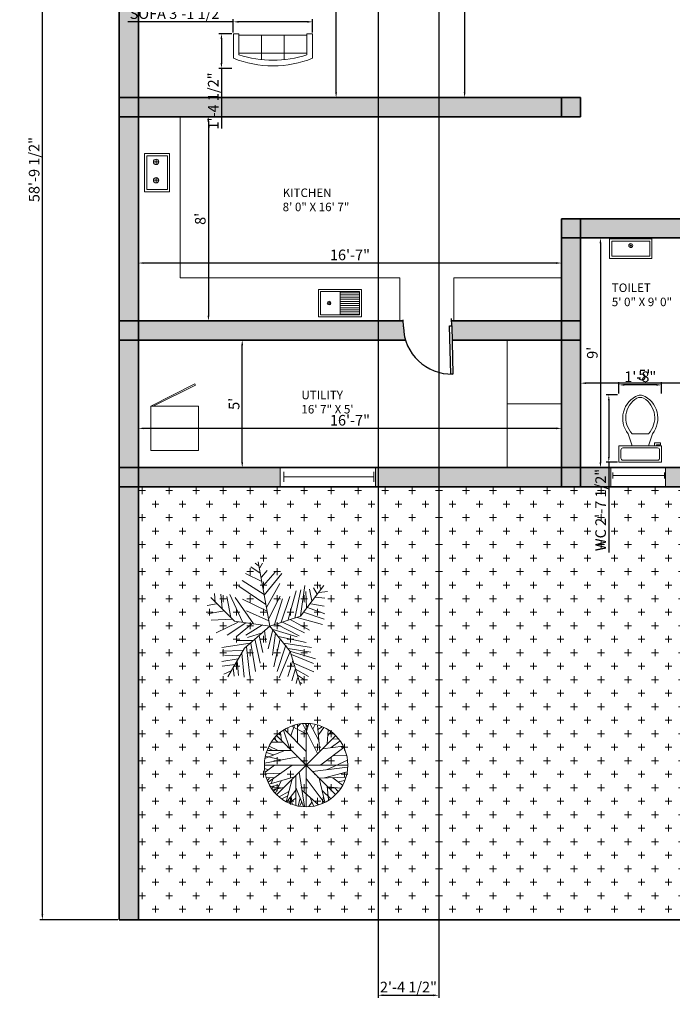
# Model space of a CAD drawing. Units: millimetres. Extents: x 2768 to 4359, y 795 to 1583.
# Tile 6 of 13: x 3572 to 3880, y 795 to 1258. Entities that reach past the tile are written whole.
import ezdxf

# ---------------------------------------------------------------- set-up
doc = ezdxf.new("R2010")
doc.units = ezdxf.units.MM
for name, color, linetype, lineweight in [('A-ANNO-DIMS', 90, 'Continuous', 18), ('A-AREA-IDEN', 190, 'Continuous', 18), ('A-EQPM', 50, 'Continuous', 18), ('A-FLOR-CASE', 50, 'Continuous', 18), ('A-FLOR-FIXT', 50, 'Continuous', 18), ('A-FLOR-FIXT-PATT', 50, 'Continuous', 13), ('A-WALL-PATT', 140, 'Continuous', 9), ('doors', 10, 'Continuous', 25), ('furniture', 50, 'Continuous', 18), ('GARDEN', 109, 'Continuous', 18), ('L-PLNT-PATT', 109, 'Continuous', 13), ('walls', 140, 'Continuous', 35), ('windows', 30, 'Continuous', 18)]:
    doc.layers.add(name, color=color, linetype=linetype, lineweight=lineweight)
doc.styles.get("Standard").update_dxf_attribs({"font": 'arial.ttf'})
doc.dimstyles.new('ISO-25', dxfattribs={"dimtxt": 5, "dimasz": 2.5, "dimexe": 1.25, "dimexo": 0.625, "dimtad": 1, "dimdec": 0, "dimlunit": 3, "dimtxsty": 'Standard', "dimcen": 2.5, "dimadec": 0, "dimazin": 0, "dimtfac": 1, "dimtdec": 0, "dimtmove": 0, "dimatfit": 3, "dimfxl": 1, "dimarcsym": 0})

# ---------------------------------------------------------------- blocks, each defined once
blk = doc.blocks.new('*U38')
for p, q in [((0, 4), (0, 0)), ((0, 2), (36, 2)), ((36, 4), (36, 0))]:
    blk.add_line(p, q)
blk = doc.blocks.new('*U39')
for p, q in [((0, 4), (0, 0)), ((36, 4), (36, 0)), ((0, 2), (36, 2))]:
    blk.add_line(p, q)
blk = doc.blocks.new('Sofa - Roundback 7 ft.')
for p, q in [((-12.00002, -32.4421), (-12.00003, -6.5971)), ((11.99997, -32.4421), (11.99998, -6.5971)), ((-36.000027, -34), (-36.000027, -11.4696)), ((-35.999844, -13.3819), (35.9998, -13.3819)), ((35.99998, -34), (35.99998, -11.4696)), ((-36.000027, -32.4421), (35.99998, -32.4421))]:
    blk.add_line(p, q)
for points in [[(-36.000027, -34), (-42.000027, -34), (-42.000027, -8)], [(41.99998, -8), (41.99998, -34), (35.99998, -34)]]:
    blk.add_lwpolyline(points)
for centre, radius, start, end in [((0, -114.25), 114.25, 68.43141, 111.5686), ((-0.00001, -127.1968), 121.1968, 72.72033, 107.2797)]:
    blk.add_arc(centre, radius, start, end)
blk = doc.blocks.new('Toilet - top')
for p, q in [((9.5, -6), (9.5, -2)), ((-10, -8.5), (-8, -8.5)), ((-10, -9.5), (-10, -8.5)), ((-7, -9.5), (-10, -9.5)), ((-8, -8.5), (-8, -8)), ((-7, -8), (-7, -9.5)), ((-4, -8), (-6, -14)), ((4, -8), (6, -14)), ((4, -14), (-4, -14))]:
    blk.add_line(p, q)
blk.add_lwpolyline([(10.5, -8), (10.5, 0), (-10.5, 0), (-10.5, -8)], close=True)
for points in [[(-9.5, -2), (-9.5, -6)], [(8.5, -1), (-8.5, -1)], [(-8.5, -7), (8.5, -7)]]:
    blk.add_lwpolyline(points)
for centre, radius, start, end in [((-8.62, -1.88), 0.884, 81.8699, 188.1301), ((8.62, -1.88), 0.884, 351.8699, 98.1301), ((-8.62, -6.12), 0.884, 171.8699, 278.1301), ((8.62, -6.12), 0.884, 261.8699, 8.1301), ((3.52, -21.58), 12.17, 141.4691, 247.9714), ((4.2, -21.82), 11.33, 136.3677, 238.9468), ((-3.52, -21.58), 12.17, 292.0284, 38.5307), ((-4.2, -21.82), 11.33, 301.053, 43.6321), ((0, -27.88), 4, 245.7318, 294.2682), ((0, -29), 4, 254.8605, 285.1395)]:
    blk.add_arc(centre, radius, start, end)
blk = doc.blocks.new('*U2')
for p, q in [((0, 0), (0, -6)), ((40, 0), (40, -6))]:
    blk.add_line(p, q)
blk.add_lwpolyline([(0, 0), (0, 40), (1.75, 40), (1.75, 0)], close=True)
blk.add_arc((0, 0), 40, 0, 90)
blk = doc.blocks.new('*D50')
at = {"layer": 'A-ANNO-DIMS', "color": 0, "lineweight": -2, "transparency": 16777216}
for p, q in [((3727.24, 1378.81), (3720.1, 1378.81)), ((3721.35, 1224.31), (3721.35, 1376.31)), ((3727.24, 1221.81), (3720.1, 1221.81))]:
    blk.add_line(p, q, dxfattribs=at)
at = {"layer": 'A-ANNO-DIMS', "color": 0, "transparency": 16777216}
for points in [[(3720.94, 1376.31), (3721.77, 1376.31), (3721.35, 1378.81)], [(3720.94, 1224.31), (3721.77, 1224.31), (3721.35, 1221.81)]]:
    blk.add_solid(points, dxfattribs=at)
at = {"layer": 'Defpoints', "color": 0, "transparency": 16777216}
for p in [(3721.35, 1378.81), (3727.87, 1378.81), (3727.87, 1221.81)]:
    blk.add_point(p, dxfattribs=at)
at = {"layer": 'A-ANNO-DIMS', "color": 0, "transparency": 16777216, "insert": (3718.17, 1300.31), "char_height": 5, "attachment_point": 5, "rotation": 90}
blk.add_mtext('13\'-1"', dxfattribs=at)
blk = doc.blocks.new('*D51')
at = {"layer": 'A-ANNO-DIMS', "color": 0, "lineweight": -2, "transparency": 16777216}
for p, q in [((3628.37, 1143.84), (3628.37, 1142.77)), ((3824.87, 1144.02), (3630.87, 1144.02)), ((3827.37, 1143.84), (3827.37, 1142.77))]:
    blk.add_line(p, q, dxfattribs=at)
at = {"layer": 'A-ANNO-DIMS', "color": 0, "transparency": 16777216}
for points in [[(3630.87, 1144.44), (3630.87, 1143.61), (3628.37, 1144.02)], [(3824.87, 1144.44), (3824.87, 1143.61), (3827.37, 1144.02)]]:
    blk.add_solid(points, dxfattribs=at)
at = {"layer": 'Defpoints', "color": 0, "transparency": 16777216}
for p in [(3628.37, 1144.47), (3628.37, 1144.02), (3827.37, 1144.47)]:
    blk.add_point(p, dxfattribs=at)
at = {"layer": 'A-ANNO-DIMS', "color": 0, "transparency": 16777216, "insert": (3727.87, 1147.2), "char_height": 5, "attachment_point": 5}
blk.add_mtext('16\'-7"', dxfattribs=at)
blk = doc.blocks.new('*D52')
at = {"layer": 'A-ANNO-DIMS', "color": 0, "lineweight": -2, "transparency": 16777216}
for p, q in [((3661.29, 1210.31), (3661.29, 1119.31)), ((3661.92, 1212.81), (3662.54, 1212.81)), ((3661.92, 1116.81), (3662.54, 1116.81))]:
    blk.add_line(p, q, dxfattribs=at)
at = {"layer": 'A-ANNO-DIMS', "color": 0, "transparency": 16777216}
for points in [[(3660.87, 1210.31), (3661.71, 1210.31), (3661.29, 1212.81)], [(3660.87, 1119.31), (3661.71, 1119.31), (3661.29, 1116.81)]]:
    blk.add_solid(points, dxfattribs=at)
at = {"layer": 'Defpoints', "color": 0, "transparency": 16777216}
for p in [(3661.29, 1212.81), (3661.29, 1116.81), (3661.29, 1116.81)]:
    blk.add_point(p, dxfattribs=at)
at = {"layer": 'A-ANNO-DIMS', "color": 0, "transparency": 16777216, "insert": (3658.11, 1164.81), "char_height": 5, "attachment_point": 5, "rotation": 90}
blk.add_mtext("8'", dxfattribs=at)
blk = doc.blocks.new('*D53')
at = {"layer": 'A-ANNO-DIMS', "color": 0, "lineweight": -2, "transparency": 16777216}
for p, q in [((3678.21, 1107.81), (3675.93, 1107.81)), ((3677.18, 1050.31), (3677.18, 1105.31)), ((3678.21, 1047.81), (3675.93, 1047.81))]:
    blk.add_line(p, q, dxfattribs=at)
at = {"layer": 'A-ANNO-DIMS', "color": 0, "transparency": 16777216}
for points in [[(3676.76, 1105.31), (3677.6, 1105.31), (3677.18, 1107.81)], [(3676.76, 1050.31), (3677.6, 1050.31), (3677.18, 1047.81)]]:
    blk.add_solid(points, dxfattribs=at)
at = {"layer": 'Defpoints', "color": 0, "transparency": 16777216}
for p in [(3677.18, 1107.81), (3678.84, 1107.81), (3678.84, 1047.81)]:
    blk.add_point(p, dxfattribs=at)
at = {"layer": 'A-ANNO-DIMS', "color": 0, "transparency": 16777216, "insert": (3674.01, 1077.81), "char_height": 5, "attachment_point": 5, "rotation": 90}
blk.add_mtext("5'", dxfattribs=at)
blk = doc.blocks.new('*D54')
at = {"layer": 'A-ANNO-DIMS', "color": 0, "lineweight": -2, "transparency": 16777216}
for p, q in [((3628.37, 1062.14), (3628.37, 1067.52)), ((3824.87, 1066.27), (3630.87, 1066.27)), ((3827.37, 1062.14), (3827.37, 1067.52))]:
    blk.add_line(p, q, dxfattribs=at)
at = {"layer": 'A-ANNO-DIMS', "color": 0, "transparency": 16777216}
for points in [[(3630.87, 1066.69), (3630.87, 1065.85), (3628.37, 1066.27)], [(3824.87, 1066.69), (3824.87, 1065.85), (3827.37, 1066.27)]]:
    blk.add_solid(points, dxfattribs=at)
at = {"layer": 'Defpoints', "color": 0, "transparency": 16777216}
for p in [(3628.37, 1066.27), (3628.37, 1061.52), (3827.37, 1061.52)]:
    blk.add_point(p, dxfattribs=at)
at = {"layer": 'A-ANNO-DIMS', "color": 0, "transparency": 16777216, "insert": (3727.87, 1069.45), "char_height": 5, "attachment_point": 5}
blk.add_mtext('16\'-7"', dxfattribs=at)
blk = doc.blocks.new('*D55')
at = {"layer": 'A-ANNO-DIMS', "color": 0, "lineweight": -2, "transparency": 16777216}
for p, q in [((3843.53, 1155.81), (3846.96, 1155.81)), ((3845.71, 1153.31), (3845.71, 1050.31)), ((3843.53, 1047.81), (3846.96, 1047.81))]:
    blk.add_line(p, q, dxfattribs=at)
at = {"layer": 'A-ANNO-DIMS', "color": 0, "transparency": 16777216}
for points in [[(3845.29, 1153.31), (3846.13, 1153.31), (3845.71, 1155.81)], [(3845.29, 1050.31), (3846.13, 1050.31), (3845.71, 1047.81)]]:
    blk.add_solid(points, dxfattribs=at)
at = {"layer": 'Defpoints', "color": 0, "transparency": 16777216}
for p in [(3842.9, 1155.81), (3842.9, 1047.81), (3845.71, 1047.81)]:
    blk.add_point(p, dxfattribs=at)
at = {"layer": 'A-ANNO-DIMS', "color": 0, "transparency": 16777216, "insert": (3842.53, 1101.81), "char_height": 5, "attachment_point": 5, "rotation": 90}
blk.add_mtext("9'", dxfattribs=at)
blk = doc.blocks.new('*D56')
at = {"layer": 'A-ANNO-DIMS', "color": 0, "lineweight": -2, "transparency": 16777216}
for p, q in [((3836.37, 1089), (3836.37, 1086.28)), ((3896.37, 1089), (3896.37, 1086.28)), ((3893.87, 1087.53), (3838.87, 1087.53))]:
    blk.add_line(p, q, dxfattribs=at)
at = {"layer": 'A-ANNO-DIMS', "color": 0, "transparency": 16777216}
for points in [[(3838.87, 1087.95), (3838.87, 1087.12), (3836.37, 1087.53)], [(3893.87, 1087.95), (3893.87, 1087.12), (3896.37, 1087.53)]]:
    blk.add_solid(points, dxfattribs=at)
at = {"layer": 'Defpoints', "color": 0, "transparency": 16777216}
for p in [(3836.37, 1089.62), (3896.37, 1089.62), (3836.37, 1087.53)]:
    blk.add_point(p, dxfattribs=at)
at = {"layer": 'A-ANNO-DIMS', "color": 0, "transparency": 16777216, "insert": (3866.37, 1090.7), "char_height": 5, "attachment_point": 5}
blk.add_mtext("5'", dxfattribs=at)
blk = doc.blocks.new('*D65')
at = {"layer": 'A-ANNO-DIMS', "color": 0, "lineweight": -2, "transparency": 16777216}
for p, q in [((3776.14, 1378.81), (3783.06, 1378.81)), ((3781.81, 1376.31), (3781.81, 1224.31)), ((3776.14, 1221.81), (3783.06, 1221.81))]:
    blk.add_line(p, q, dxfattribs=at)
at = {"layer": 'A-ANNO-DIMS', "color": 0, "transparency": 16777216}
for points in [[(3781.39, 1376.31), (3782.23, 1376.31), (3781.81, 1378.81)], [(3781.39, 1224.31), (3782.23, 1224.31), (3781.81, 1221.81)]]:
    blk.add_solid(points, dxfattribs=at)
at = {"layer": 'Defpoints', "color": 0, "transparency": 16777216}
for p in [(3775.51, 1378.81), (3775.51, 1221.81), (3781.81, 1221.81)]:
    blk.add_point(p, dxfattribs=at)
at = {"layer": 'A-ANNO-DIMS', "color": 0, "transparency": 16777216, "insert": (3778.63, 1300.31), "char_height": 5, "attachment_point": 5, "rotation": 90}
blk.add_mtext('13\'-1"', dxfattribs=at)
blk = doc.blocks.new('*U70')
for p, q in [((-8.737, 47.138), (-17.069, 52.711)), ((-10.186, 53.64), (-13.084, 55.962)), ((0, 0), (-10.5, 57)), ((-9.099, 51.782), (-6.563, 55.962)), ((-7.288, 39.707), (-21.778, 46.673)), ((-7.65, 43.423), (-2.578, 49.46)), ((-5.839, 35.992), (4.667, 48.067)), ((-5.114, 27.632), (10.463, 46.673)), ((-3.665, 19.273), (-27.574, 35.527)), ((-5.114, 28.097), (-24.676, 40.636)), ((-2.941, 16.486), (8.652, 37.85)), ((27, 9), (48, 36)), ((27.127, 9.056), (31.112, 35.992)), ((44.153, 36.456), (45.239, 32.741)), ((-48.585, 21.131), (-49.309, 29.026)), ((-43.513, 28.561), (-42.427, 15.558)), ((-38.442, 26.239), (-34.819, 7.663)), ((-35.544, 28.097), (-24.314, 3.947)), ((-1.129, 6.734), (9.014, 26.704)), ((10.101, 3.483), (17.708, 26.239)), ((16.259, 5.805), (23.142, 31.348)), ((22.055, 7.198), (27.489, 32.277)), ((31.836, 30.883), (32.561, 16.486)), ((35.096, 32.741), (37.27, 22.524)), ((38.719, 34.134), (41.979, 28.561)), ((43.791, 29.954), (51.036, 30.883)), ((-47.498, 19.737), (-55.83, 18.344)), ((-31.5, 4.5), (-52.5, 25.5)), ((-14.533, 2.09), (-30.834, 25.31)), ((-24.314, 23.917), (-2.941, 13.7)), ((3.942, 1.625), (11.187, 24.381)), ((36.183, 19.737), (48.137, 17.88)), ((40.53, 25.775), (48.862, 24.846)), ((-40.615, 13.7), (-55.105, 10.913)), ((-20.691, 13.7), (-1.129, 4.876)), ((0, 0), (27, 9)), ((29.662, 12.307), (48.137, 6.269)), ((33.285, 16.486), (48.862, 10.913)), ((-33.37, 6.269), (-52.207, 5.34)), ((-28.299, 3.483), (-47.86, -5.805)), ((-21.416, 3.018), (-38.079, -8.128)), ((0, 0), (-31.5, 4.5)), ((-15.982, 2.09), (-30.11, -9.521)), ((0, 0), (-22.5, -19.5)), ((-6.563, 1.161), (-21.416, -8.128)), ((0, 0), (18, -22.5)), ((6.478, 1.625), (26.04, -8.592)), ((11.187, 3.483), (30.749, -5.805)), ((18.07, 5.805), (35.096, -3.483)), ((24.229, 7.663), (46.688, 1.625)), ((-6.563, -5.805), (-19.967, -9.985)), ((-9.461, -8.592), (-6.201, -23.453)), ((-4.752, -3.483), (-3.665, -14.629)), ((2.493, -3.019), (-1.491, -20.202)), ((1.769, -2.555), (24.229, -9.521)), ((5.029, -6.27), (2.131, -25.775)), ((-17.431, -15.094), (-42.789, -18.809)), ((-15.257, -12.772), (-30.11, -12.772)), ((-17.069, -15.094), (-12.721, -40.172)), ((-13.446, -11.378), (-8.737, -32.741)), ((9.014, -11.378), (3.58, -35.992)), ((14.085, -16.951), (6.478, -40.172)), ((7.565, -9.056), (32.198, -14.629)), ((12.274, -15.094), (36.907, -18.809)), ((-24.314, -21.596), (-42.427, -22.06)), ((-26.849, -26.24), (-40.253, -25.775)), ((-22.5, -19.5), (-37.5, -45)), ((-25.038, -23.918), (-22.865, -45.281)), ((-20.691, -18.345), (-17.793, -44.352)), ((18.07, -22.524), (8.289, -45.745)), ((16.259, -19.738), (36.183, -22.989)), ((18, -22.5), (27, -52.5)), ((18.433, -22.524), (40.53, -29.026)), ((19.157, -25.311), (38.719, -33.206)), ((-28.299, -29.026), (-42.789, -31.348)), ((-30.834, -34.135), (-42.427, -35.528)), ((-29.023, -30.884), (-27.936, -43.887)), ((20.244, -30.419), (15.897, -44.816)), ((21.331, -32.741), (39.081, -40.636)), ((-34.457, -39.708), (-40.978, -42.494)), ((-32.646, -36.921), (-31.921, -44.352)), ((22.78, -37.85), (19.519, -48.532)), ((22.78, -38.314), (34.372, -44.816)), ((24.591, -43.423), (30.749, -47.603)), ((24.591, -45.745), (23.142, -50.854)), ((26.764, -49.925), (28.213, -50.854))]:
    blk.add_line(p, q)
blk = doc.blocks.new('*U71')
for p, q in [((-22.0458, 42.0753), (-16.5881, 57.6486)), ((-12.5388, 54.9406), (-7.9613, 59.4546)), ((-12.3627, 32.1443), (-12.5388, 58.7776)), ((-5.3205, 59.6806), (16.5105, 16.7963)), ((2.426, 54.9406), (-1.4472, 59.9056)), ((0, 59.9996), (0, -60)), ((0.4894, 48.6208), (3.6584, 59.6806)), ((18.2711, 35.5298), (5.419, 59.6806)), ((9.8203, 51.5549), (12.8133, 58.5516)), ((19.6795, 19.5047), (16.3344, 57.6486)), ((-40.1797, 44.558), (-36.4825, 43.2038)), ((-37.0107, 47.0408), (-35.25, 35.5298)), ((-32.6092, 50.4264), (-23.2782, 23.5674)), ((-31.2008, 51.1035), (-0.2149, 20.1818)), ((-26.4472, 46.5894), (-26.2712, 53.8116)), ((-21.1656, 55.8436), (-0.0388, 45.0094)), ((17.0387, 51.1035), (23.2006, 55.1666)), ((17.7429, 43.6552), (25.4894, 54.2636)), ((31.6513, 50.8778), (30.2429, 30.5643)), ((31.1232, 42.5267), (35.8767, 48.1693)), ((-49.8627, 32.8214), (-32.7853, 32.8214)), ((-45.8134, 38.2383), (-40.5318, 33.0471)), ((-43.8768, 36.4326), (-44.405, 40.2696)), ((42, 42), (-42, -42)), ((42, -42), (-42, 42)), ((36.2288, 25.1474), (48.9049, 35.0784)), ((37.1091, 37.1098), (46.6161, 37.5612)), ((-32.2571, 20.6333), (-59.1937, 9.348)), ((-57.081, 17.9248), (-47.0458, 14.7649)), ((-56.0247, 20.859), (-20.8134, 20.859)), ((-54.7923, 24.4702), (-47.75, 21.0847)), ((-53.2078, 27.4044), (-40.1797, 20.859)), ((54.3626, 25.3731), (20.9119, 0.3198)), ((23.3767, 23.3417), (53.3063, 27.4044)), ((-59.7219, 2.8025), (-12.0106, 12.0565)), ((-58.6656, 12.7336), (-35.9543, 7.5424)), ((-54.6162, -24.7335), (-20.2853, 0.0941)), ((29.3626, -6.6771), (59.4682, 7.091)), ((38.5175, 13.4107), (58.2359, 13.6364)), ((-60, 0), (60, 0)), ((-59.7219, -4.8714), (-54.2641, -6.6771)), ((-45.2853, -0.1316), (-59.0177, -10.0627)), ((-58.4895, -12.3197), (-36.4825, -11.6426)), ((-10.074, -10.0627), (-2.5036, -59.7178)), ((9.2922, -9.1598), (59.6443, -2.8401)), ((26.3697, -18.4138), (58.9401, -9.8369)), ((-57.081, -18.4138), (-45.2853, -17.9624)), ((-52.6797, -18.188), (-55.4966, -22.0251)), ((-53.2078, -27.442), (-16.7641, -16.6081)), ((-47.2219, -19.3166), (-50.2148, -26.3135)), ((-35.9543, -22.4765), (-44.0529, -40.5329)), ((-19.9331, -20.2194), (-28.5599, -52.721)), ((-14.8275, -15.0282), (-14.6515, -57.6865)), ((-0.0388, -19.0909), (25.8415, -53.8495)), ((18.6232, -18.6394), (26.7218, -53.3981)), ((18.7992, -18.6394), (57.3556, -17.2853)), ((38.1654, -18.188), (52.426, -29.0219)), ((45.9119, -24.0564), (55.595, -22.2508)), ((-38.9472, -29.0219), (-51.4472, -30.6018)), ((-46.5177, -30.1504), (-49.5106, -33.536)), ((-32.4331, -32.4075), (-48.1021, -35.5674)), ((-43.7008, -34.6645), (-46.6937, -37.373)), ((-24.6867, -37.8244), (-38.7712, -45.7241)), ((-14.6515, -36.2445), (-27.6797, -52.9467)), ((-14.6515, -32.1818), (-3.912, -59.4922)), ((-6.2008, -36.2445), (17.919, -57.0094)), ((22.8485, -36.4702), (35.3485, -48.4326)), ((30.419, -30.1504), (32.3556, -50.0125)), ((31.4753, -31.279), (49.6091, -33.3103)), ((41.5105, -32.6332), (46.088, -38.0501)), ((-26.2712, -43.9185), (-34.7219, -48.6583)), ((-14.6515, -47.3041), (-25.0388, -54.3009)), ((-21.5177, -45.4984), (-19.9331, -56.1065)), ((-8.4895, -47.5298), (-11.4825, -58.5893)), ((-6.3768, -52.721), (-9.3698, -58.815)), ((8.4119, -53.1724), (3.8344, -59.4922)), ((5.9471, -46.6269), (10.5246, -58.5893)), ((24.7852, -44.8213), (23.0246, -54.978))]:
    blk.add_line(p, q)
blk.add_circle((0, 0), 60)
blk = doc.blocks.new('*D79')
at = {"layer": 'A-ANNO-DIMS', "color": 0, "lineweight": -2, "transparency": 16777216}
for p, q in [((3853.76, 1081.98), (3848.4, 1081.98)), ((3849.65, 1079.48), (3849.65, 1052.86)), ((3853.76, 1050.36), (3848.4, 1050.36)), ((3849.65, 1050.36), (3849.65, 1007.88))]:
    blk.add_line(p, q, dxfattribs=at)
at = {"layer": 'A-ANNO-DIMS', "color": 0, "transparency": 16777216}
for points in [[(3849.23, 1079.48), (3850.06, 1079.48), (3849.65, 1081.98)], [(3849.23, 1052.86), (3850.06, 1052.86), (3849.65, 1050.36)]]:
    blk.add_solid(points, dxfattribs=at)
at = {"layer": 'Defpoints', "color": 0, "transparency": 16777216}
for p in [(3854.39, 1081.98), (3849.65, 1050.36), (3854.39, 1050.36)]:
    blk.add_point(p, dxfattribs=at)
at = {"layer": 'A-ANNO-DIMS', "color": 0, "transparency": 16777216, "insert": (3846.44, 1027.87), "char_height": 5, "attachment_point": 5, "rotation": 90}
blk.add_mtext('WC 2\'-7 1/2"', dxfattribs=at)
blk = doc.blocks.new('*D80')
at = {"layer": 'A-ANNO-DIMS', "color": 0, "lineweight": -2, "transparency": 16777216}
for p, q in [((3854.39, 1082.6), (3854.39, 1087.97)), ((3871.98, 1086.72), (3856.89, 1086.72)), ((3874.48, 1082.6), (3874.48, 1087.97))]:
    blk.add_line(p, q, dxfattribs=at)
at = {"layer": 'A-ANNO-DIMS', "color": 0, "transparency": 16777216}
for points in [[(3856.89, 1087.14), (3856.89, 1086.3), (3854.39, 1086.72)], [(3871.98, 1087.14), (3871.98, 1086.3), (3874.48, 1086.72)]]:
    blk.add_solid(points, dxfattribs=at)
at = {"layer": 'Defpoints', "color": 0, "transparency": 16777216}
for p in [(3854.39, 1086.72), (3854.39, 1081.98), (3874.48, 1081.98)]:
    blk.add_point(p, dxfattribs=at)
at = {"layer": 'A-ANNO-DIMS', "color": 0, "transparency": 16777216, "insert": (3864.44, 1089.9), "char_height": 5, "attachment_point": 5}
blk.add_mtext('1\'-8"', dxfattribs=at)
blk = doc.blocks.new('*D105')
at = {"layer": 'A-ANNO-DIMS', "color": 0, "lineweight": -2, "transparency": 16777216}
for p, q in [((3673, 1257.45), (3623.37, 1257.45)), ((3673, 1252.49), (3673, 1258.7)), ((3707.79, 1257.45), (3675.5, 1257.45)), ((3710.29, 1252.49), (3710.29, 1258.7))]:
    blk.add_line(p, q, dxfattribs=at)
at = {"layer": 'A-ANNO-DIMS', "color": 0, "transparency": 16777216}
for points in [[(3675.5, 1257.87), (3675.5, 1257.04), (3673, 1257.45)], [(3707.79, 1257.87), (3707.79, 1257.04), (3710.29, 1257.45)]]:
    blk.add_solid(points, dxfattribs=at)
at = {"layer": 'Defpoints', "color": 0, "transparency": 16777216}
for p in [(3673, 1257.45), (3673, 1251.86), (3710.29, 1251.86)]:
    blk.add_point(p, dxfattribs=at)
at = {"layer": 'A-ANNO-DIMS', "color": 0, "transparency": 16777216, "insert": (3646.94, 1260.67), "char_height": 5, "attachment_point": 5}
blk.add_mtext('SOFA 3\'-1 1/2"', dxfattribs=at)
blk = doc.blocks.new('*D106')
at = {"layer": 'A-ANNO-DIMS', "color": 0, "lineweight": -2, "transparency": 16777216}
for p, q in [((3672.37, 1251.86), (3666.16, 1251.86)), ((3667.41, 1249.36), (3667.41, 1238.08)), ((3672.37, 1235.58), (3666.16, 1235.58)), ((3667.41, 1235.58), (3667.41, 1207.36))]:
    blk.add_line(p, q, dxfattribs=at)
at = {"layer": 'A-ANNO-DIMS', "color": 0, "transparency": 16777216}
for points in [[(3666.99, 1249.36), (3667.82, 1249.36), (3667.41, 1251.86)], [(3666.99, 1238.08), (3667.82, 1238.08), (3667.41, 1235.58)]]:
    blk.add_solid(points, dxfattribs=at)
at = {"layer": 'Defpoints', "color": 0, "transparency": 16777216}
for p in [(3673, 1251.86), (3667.41, 1235.58), (3673, 1235.58)]:
    blk.add_point(p, dxfattribs=at)
at = {"layer": 'A-ANNO-DIMS', "color": 0, "transparency": 16777216, "insert": (3664.2, 1220.22), "char_height": 5, "attachment_point": 5, "rotation": 90}
blk.add_mtext('1\'-4 1/2"', dxfattribs=at)
blk = doc.blocks.new('*D129')
at = {"layer": 'A-ANNO-DIMS', "color": 0, "lineweight": -2, "transparency": 16777216}
for p, q in [((3618.74, 1540.81), (3581.91, 1540.81)), ((3583.16, 837.66), (3583.16, 1538.31)), ((3618.74, 835.16), (3581.91, 835.16))]:
    blk.add_line(p, q, dxfattribs=at)
at = {"layer": 'A-ANNO-DIMS', "color": 0, "transparency": 16777216}
for points in [[(3582.75, 1538.31), (3583.58, 1538.31), (3583.16, 1540.81)], [(3582.75, 837.66), (3583.58, 837.66), (3583.16, 835.16)]]:
    blk.add_solid(points, dxfattribs=at)
at = {"layer": 'Defpoints', "color": 0, "transparency": 16777216}
for p in [(3583.16, 1540.81), (3619.37, 1540.81), (3619.37, 835.16)]:
    blk.add_point(p, dxfattribs=at)
at = {"layer": 'A-ANNO-DIMS', "color": 0, "transparency": 16777216, "insert": (3579.95, 1187.98), "char_height": 5, "attachment_point": 5, "rotation": 90}
blk.add_mtext('58\'-9 1/2"', dxfattribs=at)
blk = doc.blocks.new('*D135')
at = {"layer": 'A-ANNO-DIMS', "color": 0, "lineweight": -2, "transparency": 16777216}
for p, q in [((3741.08, 1378.18), (3741.08, 798.41)), ((3769.66, 1378.18), (3769.66, 798.41)), ((3743.58, 799.66), (3767.16, 799.66))]:
    blk.add_line(p, q, dxfattribs=at)
at = {"layer": 'A-ANNO-DIMS', "color": 0, "transparency": 16777216}
for points in [[(3743.58, 800.08), (3743.58, 799.24), (3741.08, 799.66)], [(3767.16, 800.08), (3767.16, 799.24), (3769.66, 799.66)]]:
    blk.add_solid(points, dxfattribs=at)
at = {"layer": 'Defpoints', "color": 0, "transparency": 16777216}
for p in [(3741.08, 1378.81), (3769.66, 1378.81), (3769.66, 799.66)]:
    blk.add_point(p, dxfattribs=at)
at = {"layer": 'A-ANNO-DIMS', "color": 0, "transparency": 16777216, "insert": (3755.37, 802.87), "char_height": 5, "attachment_point": 5}
blk.add_mtext('2\'-4 1/2"', dxfattribs=at)

msp = doc.modelspace()

# ---------------------------------------------------------------- hatches: boundary and pattern name
at = {"layer": 'A-FLOR-FIXT-PATT'}
h = msp.add_hatch(dxfattribs=at)
h.set_pattern_fill('ANSI31', color=256, scale=0.3149606, angle=-45, style=0)
h.paths.add_polyline_path([(3723.19, 1119.71), (3732.34, 1119.71), (3732.34, 1130.65), (3723.19, 1130.65)])
at = {"layer": 'A-WALL-PATT'}
h = msp.add_hatch(color=256, dxfattribs=at)
h.dxf.hatch_style = 1
h.paths.add_polyline_path([(3666.8, 1540.81), (3628.37, 1540.81), (3628.37, 1531.81), (3666.8, 1531.81)])
h.paths.add_polyline_path([(3628.37, 1540.81), (3619.37, 1540.81), (3619.37, 1531.81), (3628.37, 1531.81)])
h.paths.add_polyline_path([(3628.37, 1531.81), (3619.37, 1531.81), (3619.37, 1387.81), (3628.37, 1387.81)])
h.paths.add_polyline_path([(3772.37, 1540.81), (3710.62, 1540.81), (3710.62, 1531.81), (3772.37, 1531.81)])
h.paths.add_polyline_path([(3796.31, 1540.81), (3781.37, 1540.81), (3781.37, 1531.81), (3796.31, 1531.81)])
h.paths.add_polyline_path([(3781.37, 1540.81), (3772.37, 1540.81), (3772.37, 1531.81), (3781.37, 1531.81)])
h.paths.add_polyline_path([(3781.37, 1531.81), (3772.37, 1531.81), (3772.37, 1493.05), (3773.51, 1493.08), (3781.37, 1493.27)])
h.paths.add_polyline_path([(3841.37, 1540.81), (3822.12, 1540.81), (3822.12, 1531.81), (3841.37, 1531.81)])
h.paths.add_polyline_path([(3867.29, 1540.81), (3850.37, 1540.81), (3850.37, 1531.81), (3867.29, 1531.81)])
h.paths.add_polyline_path([(3850.37, 1540.81), (3841.37, 1540.81), (3841.37, 1531.81), (3850.37, 1531.81)])
h.paths.add_polyline_path([(3850.37, 1531.81), (3841.37, 1531.81), (3841.37, 1435.81), (3850.37, 1435.81)])
h.paths.add_polyline_path([(3919.37, 1531.81), (3910.37, 1531.81), (3910.37, 1495.39, -0.097322), (3918.93, 1497.3), (3919.37, 1497.31)])
h.paths.add_polyline_path([(3919.37, 1540.81), (3910.37, 1540.81), (3910.37, 1531.81), (3919.37, 1531.81)])
h.paths.add_polyline_path([(3910.37, 1540.81), (3893.19, 1540.81), (3893.19, 1531.81), (3910.37, 1531.81)])
h.paths.add_polyline_path([(3971.85, 1540.81), (3919.37, 1540.81), (3919.37, 1531.81), (3971.85, 1531.81)])
h.paths.add_polyline_path([(4063.37, 1540.81), (4017.44, 1540.81), (4017.44, 1531.81), (4063.37, 1531.81)])
h.paths.add_polyline_path([(4072.37, 1531.81), (4063.37, 1531.81), (4063.37, 1387.81), (4072.37, 1387.81)])
h.paths.add_polyline_path([(4072.37, 1378.81), (4063.37, 1378.81), (4063.37, 1240.81), (4072.37, 1240.81)])
h.paths.add_polyline_path([(4072.37, 1387.81), (4063.37, 1387.81), (4063.37, 1378.81), (4072.37, 1378.81)])
h.paths.add_polyline_path([(3919.37, 1387.81), (3910.37, 1387.81), (3910.37, 1378.81), (3919.37, 1378.81)])
h.paths.add_polyline_path([(3919.37, 1392.95, -0.05459), (3913.18, 1392.28), (3910.37, 1392.28), (3910.37, 1387.81), (3919.37, 1387.81)])
h.paths.add_polyline_path([(3919.37, 1474.55), (3910.37, 1474.32), (3910.37, 1435.81), (3919.37, 1435.81)])
h.paths.add_polyline_path([(3919.37, 1435.81), (3910.37, 1435.81), (3910.37, 1426.81), (3919.37, 1426.81)])
h.paths.add_polyline_path([(3910.37, 1435.81), (3850.37, 1435.81), (3850.37, 1426.81), (3910.37, 1426.81)])
h.paths.add_polyline_path([(3919.37, 1426.81), (3910.37, 1426.81), (3910.37, 1420.86), (3913.18, 1420.86), (3919.37, 1420.86)])
h.paths.add_polyline_path([(3850.37, 1435.81), (3841.37, 1435.81), (3841.37, 1426.81), (3850.37, 1426.81)])
h.paths.add_polyline_path([(3841.37, 1435.81), (3781.37, 1435.81), (3781.37, 1426.81), (3841.37, 1426.81)])
h.paths.add_polyline_path([(3781.37, 1435.81), (3772.37, 1435.81), (3772.37, 1426.81), (3781.37, 1426.81)])
h.paths.add_polyline_path([(3781.37, 1426.81), (3772.37, 1426.81), (3772.37, 1420.59, -0.050492), (3778.09, 1421.17), (3781.37, 1421.17)])
h.paths.add_polyline_path([(3781.37, 1471.72, -0.082137), (3774.07, 1470.33), (3772.37, 1470.29), (3772.37, 1435.81), (3781.37, 1435.81)])
h.paths.add_polyline_path([(3628.37, 1387.81), (3619.37, 1387.81), (3619.37, 1378.81), (3628.37, 1378.81)])
h.paths.add_polyline_path([(3628.37, 1378.81), (3619.37, 1378.81), (3619.37, 1346.39), (3622.95, 1346.39), (3628.37, 1346.39)])
h.paths.add_polyline_path([(3781.37, 1387.81), (3772.37, 1387.81), (3772.37, 1378.81), (3781.37, 1378.81)])
h.paths.add_polyline_path([(3781.37, 1392.59), (3778.09, 1392.59), (3772.37, 1392.59), (3772.37, 1387.81), (3781.37, 1387.81)])
h.paths.add_polyline_path([(3628.37, 1318.32, -0.047705), (3622.95, 1317.81), (3619.37, 1317.81), (3619.37, 1221.81), (3628.37, 1221.81)])
h.paths.add_polyline_path([(3628.37, 1221.81), (3619.37, 1221.81), (3619.37, 1212.81), (3628.37, 1212.81)])
h.paths.add_polyline_path([(3827.37, 1221.81), (3628.37, 1221.81), (3628.37, 1212.81), (3827.37, 1212.81)])
h.paths.add_polyline_path([(3628.37, 1212.81), (3619.37, 1212.81), (3619.37, 1116.81), (3628.37, 1116.81)])
h.paths.add_polyline_path([(3836.37, 1221.81), (3827.37, 1221.81), (3827.37, 1212.81), (3836.37, 1212.81)])
h.paths.add_polyline_path([(3628.37, 1107.81), (3619.37, 1107.81), (3619.37, 1047.81), (3628.37, 1047.81)])
h.paths.add_polyline_path([(3628.37, 1116.81), (3619.37, 1116.81), (3619.37, 1107.81), (3628.37, 1107.81)])
h.paths.add_polyline_path([(3836.37, 1155.81), (3827.37, 1155.81), (3827.37, 1116.81), (3836.37, 1116.81)])
h.paths.add_polyline_path([(3836.37, 1116.81), (3827.37, 1116.81), (3827.37, 1107.81), (3836.37, 1107.81)])
h.paths.add_polyline_path([(3836.37, 1107.81), (3827.37, 1107.81), (3827.37, 1047.81), (3836.37, 1047.81)])
h.paths.add_polyline_path([(3827.37, 1047.37), (3827.37, 1047.81), (3739.96, 1047.81), (3739.96, 1038.81), (3827.37, 1038.81)])
h.paths.add_polyline_path([(3836.37, 1047.37), (3836.37, 1047.81), (3827.37, 1047.81), (3827.37, 1047.37), (3827.37, 1038.81), (3836.37, 1038.81)])
h.paths.add_polyline_path([(3695.08, 1047.81), (3628.37, 1047.81), (3628.37, 1038.81), (3695.08, 1038.81)])
h.paths.add_polyline_path([(3628.37, 1047.81), (3619.37, 1047.81), (3619.37, 1038.81), (3628.37, 1038.81)])
h.paths.add_polyline_path([(3850.59, 1047.81), (3836.37, 1047.81), (3836.37, 1047.37), (3836.37, 1038.81), (3850.59, 1038.81)])
h.paths.add_polyline_path([(3896.37, 1047.37), (3896.37, 1047.81), (3876.26, 1047.81), (3876.26, 1038.81), (3896.37, 1038.81)])
h.paths.add_polyline_path([(3905.37, 1109.65), (3903.46, 1109.6), (3896.37, 1109.43), (3896.37, 1047.81), (3905.37, 1047.81)])
h.paths.add_polyline_path([(3905.37, 1047.81), (3896.37, 1047.81), (3896.37, 1047.37), (3896.37, 1038.81), (3905.37, 1038.81)])
h.paths.add_polyline_path([(4063.37, 1047.81), (3905.37, 1047.81), (3905.37, 1038.81), (4063.37, 1038.81)])
h.paths.add_polyline_path([(4072.37, 1137.28), (4063.37, 1137.28), (4063.37, 1047.81), (4072.37, 1047.81)])
h.paths.add_polyline_path([(4072.37, 1231.81), (4063.37, 1231.81), (4063.37, 1182.55), (4072.37, 1182.55)])
h.paths.add_polyline_path([(4072.37, 1240.81), (4063.37, 1240.81), (4063.37, 1231.81), (4072.37, 1231.81)])
h.paths.add_polyline_path([(4072.37, 1047.81), (4063.37, 1047.81), (4063.37, 1038.81), (4072.37, 1038.81)])
h.paths.add_polyline_path([(3905.37, 1231.81), (3896.37, 1231.81), (3896.37, 1164.81), (3905.37, 1164.81)])
h.paths.add_polyline_path([(3905.37, 1240.81), (3896.37, 1240.81), (3896.37, 1231.81), (3905.37, 1231.81)])
h.paths.add_polyline_path([(3910.61, 1237.57), (3910.61, 1240.81), (3905.37, 1240.81), (3905.37, 1231.81), (3911.2, 1231.81, -0.050754)])
h.paths.add_polyline_path([(3988.37, 1240.81), (3939.19, 1240.81), (3939.19, 1237.57), (3939.19, 1231.81), (3988.37, 1231.81)])
h.paths.add_polyline_path([(3997.37, 1240.81), (3988.37, 1240.81), (3988.37, 1231.81), (3997.37, 1231.81)])
h.paths.add_polyline_path([(4063.37, 1240.81), (3997.37, 1240.81), (3997.37, 1231.81), (4063.37, 1231.81)])
h.paths.add_polyline_path([(3997.37, 1334.21), (3988.37, 1334.21), (3988.37, 1288.44), (3997.37, 1288.44)])
h.paths.add_polyline_path([(3896.37, 1164.81), (3836.37, 1164.81), (3836.37, 1155.81), (3896.37, 1155.81)])
h.paths.add_polyline_path([(3836.37, 1164.81), (3827.37, 1164.81), (3827.37, 1155.81), (3836.37, 1155.81)])
h.paths.add_polyline_path([(3905.37, 1164.81), (3896.37, 1164.81), (3896.37, 1155.81), (3905.37, 1155.81)])
h.paths.add_polyline_path([(3905.37, 1155.81), (3896.37, 1155.81), (3896.37, 1131.22, -0.073168), (3902.89, 1132.35), (3905.37, 1132.41)])
edge = h.paths.add_edge_path()
edge.add_line((3951.89, 1380.74), (3951.89, 1378.81))
edge.add_line((3951.89, 1378.81), (4063.37, 1378.81))
edge.add_line((4063.37, 1378.81), (4063.37, 1387.81))
edge.add_line((4063.37, 1387.81), (3951, 1387.81))
edge.add_arc((3923.31, 1380.74), 28.58, 0, 14.3236, ccw=False)
h.paths.add_polyline_path([(3923.31, 1378.81), (3923.31, 1387.81), (3919.37, 1387.81), (3919.37, 1378.81)])
edge = h.paths.add_edge_path()
edge.add_arc((3775.74, 1114.53), 22.75, 187.4686, 197.1843)
edge.add_line((3754, 1107.81), (3628.37, 1107.81))
edge.add_line((3628.37, 1107.81), (3628.37, 1116.81))
edge.add_line((3628.37, 1116.81), (3752.42, 1116.81))
edge.add_arc((3775.17, 1117.41), 22.75, 181.5276, 194.8757)
h.paths.add_polyline_path([(3775.68, 1116.81), (3775.91, 1107.81), (3827.37, 1107.81), (3827.37, 1116.81)])
h = msp.add_hatch(color=256, dxfattribs=at)
h.dxf.hatch_style = 1
h.paths.add_polyline_path([(3628.37, 1038.81), (3619.37, 1038.81), (3619.37, 835.16), (3628.37, 835.16)])
h.paths.add_polyline_path([(4072.37, 1007.81), (4068.9, 1007.81), (4067.72, 1007.81), (4063.37, 1007.81), (4063.37, 835.16), (4072.37, 835.16)])
at = {"layer": 'L-PLNT-PATT'}
h = msp.add_hatch(dxfattribs=at)
h.set_pattern_fill('CROSS', color=256)
h.set_pattern_definition([(0, (-194.219, 46.374), (6.35, 6.35), [3.175, -9.525]), (90, (-192.6314, 44.7867), (-6.35, 6.35), [3.175, -9.525])])
h.paths.add_polyline_path([(3628.37, 1038.81), (3628.37, 835.16), (4063.37, 835.16), (4063.37, 1007.81), (4063.37, 1038.81), (3905.37, 1038.81), (3896.37, 1038.81)])
h.paths.add_polyline_path([(3691.58, 971.77), (3691.54, 971.61), (3692.89, 969.92), (3693.09, 971.3)], flags=16)
h.paths.add_polyline_path([(3686.64, 970.14), (3687.8, 970.5), (3687.74, 971.09)], flags=16)
h.paths.add_polyline_path([(3726.85, 906.98), (3710.25, 904.9), (3713.35, 901.8), (3715.93, 901.89), (3726.61, 904.7, 0.029207)], flags=16)
h.paths.add_polyline_path([(3703.16, 924.71), (3703.15, 925.88), (3702.38, 925.11)], flags=16)
h.paths.add_polyline_path([(3994.35, 978.45), (3994.55, 980.25), (3996.36, 982.82), (3998.16, 983.85), (3997.16, 985.65), (3994.96, 986.93), (3999.36, 986.93), (4002.17, 988.73), (3997.76, 992.07), (4000.17, 992.58), (3997.16, 995.41), (4001.97, 995.41), (4004.17, 995.93), (4004.17, 997.72), (4001.77, 1000.29), (4000.57, 1001.06), (4004.98, 1000.29), (4008.78, 999.52), (4010.59, 1001.06), (4009.99, 1003.63), (4010.39, 1005.94), (4008.98, 1008.51), (4011.79, 1006.97), (4012.79, 1003.63), (4015.6, 1001.83), (4015.8, 1003.89), (4015.4, 1005.94), (4016.6, 1008.51), (4020.61, 1007.74), (4023.21, 1005.17), (4023.61, 1006.2), (4024.54, 1010.18), (4026.42, 1012.88), (4029.22, 1009.03), (4030.23, 1011.34), (4033.23, 1007.74), (4035.84, 1011.34), (4036.24, 1007.74), (4039.44, 1009.54), (4041.45, 1013.14), (4041.25, 1007.74), (4040.45, 1005.69), (4042.85, 1006.97), (4045.06, 1008.77), (4044.25, 1005.17), (4044.05, 1003.12), (4045.46, 1002.35), (4047.46, 1004.15), (4049.06, 1005.69), (4049.46, 1003.38), (4048.26, 1000.81), (4048.06, 997.98), (4049.66, 996.95), (4052.47, 998.75), (4053.87, 999.26), (4052.47, 995.41), (4050.67, 992.84), (4050.87, 991.04), (4053.27, 990.27), (4055.88, 991.3), (4058.28, 991.3), (4056.88, 990.53), (4054.67, 989.25), (4053.27, 986.93), (4055.08, 986.42), (4057.08, 986.42), (4059.48, 986.93), (4057.88, 984.11), (4055.48, 983.08), (4053.87, 981.54), (4053.67, 979.74), (4056.08, 978.71), (4057.68, 978.2), (4060.26, 979.38), (4059.68, 977.17), (4056.88, 975.89), (4053.47, 975.63), (4052.47, 974.6), (4053.67, 972.8), (4054.88, 971.52), (4057.88, 970.49), (4061.29, 969.46), (4058.28, 968.95), (4055.68, 969.21), (4051.07, 967.15), (4052.87, 963.81), (4050.87, 964.58), (4049.06, 963.3), (4049.06, 962.01), (4051.47, 958.93), (4049.46, 959.7), (4044.86, 960.47), (4043.25, 959.19), (4043.85, 956.62), (4045.86, 952.76), (4044.86, 953.53), (4042.05, 955.85), (4038.84, 956.62), (4037.84, 955.08), (4038.44, 949.17), (4036.64, 953.28), (4035.64, 956.1), (4034.23, 957.64), (4033.23, 955.85), (4032.83, 949.17), (4031.63, 951.22), (4029.22, 952.51), (4028.82, 949.94), (4025.82, 954.05), (4025.42, 948.65), (4023.81, 955.59), (4022.81, 953.02), (4022.81, 955.08), (4020.61, 952.25), (4019.81, 950.19), (4018.2, 953.79), (4016.4, 953.53), (4015, 950.71), (4014.8, 953.79), (4013.99, 956.62), (4011.39, 957.39), (4007.78, 955.08), (4008.78, 958.16), (4009.38, 961.5), (4004.98, 962.01), (4006.18, 964.32), (4000.97, 960.21), (4003.77, 965.1), (4001.57, 964.58), (4003.77, 967.41), (4003.57, 969.21), (4000.97, 969.98), (3995.76, 968.18), (4000.57, 974.09), (3995.36, 973.06), (3998.56, 975.63), (3999.36, 978.71), (3997.76, 980.25), (3995.36, 979.23)], flags=16)
h.paths.add_polyline_path([(4026.42, 981.02), (4026.62, 982.05), (4027.62, 981.79), (4027.42, 981.28)], flags=0)

# ---------------------------------------------------------------- linework, layer by layer
at = {"layer": 'A-EQPM'}
for p, q in [((3637.93, 1191.61), (3635.39, 1191.61)), ((3636.66, 1192.89), (3636.66, 1190.34)), ((3637.93, 1182.95), (3635.39, 1182.95)), ((3636.66, 1182.95), (3636.66, 1184.22)), ((3636.66, 1184.22), (3636.66, 1181.68)), ((3634.24, 1076.69), (3654.86, 1087.28)), ((3655.25, 1086.52), (3635.34, 1076.69)), ((3654.86, 1087.28), (3655.25, 1086.52))]:
    msp.add_line(p, q, dxfattribs=at)
for points in [[(3631.28, 1195.46), (3642.96, 1195.46), (3642.96, 1177.54), (3631.28, 1177.54)], [(3632.28, 1194.46), (3641.96, 1194.46), (3641.96, 1178.54), (3632.28, 1178.54)], [(3634.24, 1055.86), (3656.6, 1055.86), (3656.6, 1076.69), (3634.24, 1076.69)]]:
    msp.add_lwpolyline(points, close=True, dxfattribs=at)
for centre in [(3636.66, 1191.61), (3636.66, 1182.95)]:
    msp.add_circle(centre, 1.27, dxfattribs=at)
at = {"layer": 'A-FLOR-CASE'}
for p, q in [((3628.37, 1212.81), (3648.02, 1212.81)), ((3648.02, 1212.81), (3648.02, 1137.11)), ((3648.02, 1137.11), (3751.26, 1137.11)), ((3751.26, 1116.81), (3751.26, 1137.11)), ((3776.71, 1137.11), (3776.71, 1116.81)), ((3776.71, 1137.11), (3827.37, 1137.11)), ((3801.9, 1077.81), (3827.37, 1077.81))]:
    msp.add_line(p, q, dxfattribs=at)
msp.add_lwpolyline([(3827.37, 1107.81), (3801.9, 1107.81), (3801.9, 1047.81), (3827.37, 1047.81)], close=True, dxfattribs=at)
at = {"layer": 'A-FLOR-FIXT'}
msp.add_line((3723.19, 1119.71), (3723.19, 1130.65), dxfattribs=at)
for points in [[(3850.04, 1155.38), (3869.87, 1155.38), (3869.87, 1146.2), (3850.04, 1146.2)], [(3851.04, 1154.38), (3868.87, 1154.38), (3868.87, 1147.2), (3851.04, 1147.2)], [(3713.03, 1131.65), (3733.34, 1131.65), (3733.34, 1118.71), (3713.03, 1118.71)], [(3714.03, 1130.65), (3732.34, 1130.65), (3732.34, 1119.71), (3714.03, 1119.71)]]:
    msp.add_lwpolyline(points, close=True, dxfattribs=at)
for centre, radius in [((3859.95, 1152.22), 0.913), ((3859.95, 1152.22), 0.337), ((3718.03, 1125.18), 0.865), ((3718.03, 1125.18), 0.423)]:
    msp.add_circle(centre, radius, dxfattribs=at)
at = {"layer": 'walls'}
for p, q in [((3619.37, 1317.81), (3619.37, 835.16)), ((3628.37, 1318.32), (3628.37, 835.16)), ((3836.37, 1221.81), (3619.37, 1221.81)), ((3827.37, 1221.81), (3827.37, 1212.81)), ((3836.37, 1221.81), (3836.37, 1212.81)), ((3836.37, 1212.81), (3619.37, 1212.81)), ((3905.37, 1164.81), (3827.37, 1164.81)), ((3827.37, 1164.81), (3827.37, 1047.37)), ((3836.37, 1164.81), (3836.37, 1047.37)), ((3905.37, 1155.81), (3827.37, 1155.81)), ((3752.92, 1116.81), (3619.37, 1116.81)), ((3836.37, 1116.81), (3775.68, 1116.81)), ((3754, 1107.81), (3619.37, 1107.81)), ((3836.37, 1107.81), (3775.91, 1107.81)), ((3896.37, 1047.81), (3619.37, 1047.81)), ((3827.37, 1047.37), (3827.37, 1038.81)), ((3836.37, 1047.37), (3836.37, 1038.81)), ((3896.37, 1038.81), (3619.37, 1038.81)), ((4072.37, 835.16), (3619.37, 835.16))]:
    msp.add_line(p, q, dxfattribs=at)
at = {"layer": 'windows'}
for p, q in [((3695.08, 1047.81), (3695.08, 1038.81)), ((3739.96, 1047.81), (3739.96, 1038.81)), ((3850.59, 1047.81), (3850.59, 1038.81)), ((3876.26, 1047.81), (3876.26, 1038.81))]:
    msp.add_line(p, q, dxfattribs=at)

# ---------------------------------------------------------------- block references
at = {"layer": 'A-FLOR-FIXT', "xscale": 0.956759624166975, "yscale": 0.956759624166975, "zscale": 0.956759624166975, "rotation": 180}
msp.add_blockref('Toilet - top', (3864.44, 1050.36), dxfattribs=at)
at = {"layer": 'doors', "xscale": 0.5688608536322607, "yscale": 0.5688608536322607, "zscale": 0.5688608536322607, "rotation": 181.4234424507562}
msp.add_blockref('*U2', (3775.74, 1114.53), dxfattribs=at)
at = {"layer": 'furniture', "xscale": 0.4439665590172627, "yscale": 0.4439665590172627, "zscale": 0.4439665590172627, "rotation": 180}
msp.add_blockref('Sofa - Roundback 7 ft.', (3691.65, 1236.77), dxfattribs=at)
at = {"layer": 'GARDEN'}
for name, p, xscale, yscale, zscale in [('*U70', (3690.23, 973.25), 0.5295290304152854, 0.5295290304152854, 0.5295290304152854), ('*U71', (3707.25, 907.9), 0.3271061411482715, 0.3271061411482715, 0.3271061411482715)]:
    msp.add_blockref(name, p, dxfattribs=dict(at, xscale=xscale, yscale=yscale, zscale=zscale))
at = {"layer": 'windows'}
for name, p, xscale, yscale, zscale in [('*U39', (3696.7, 1041.05), 1.175999919670228, 1.175999919670228, 1.175999919670228), ('*U38', (3851.49, 1042.75), 0.6767405614116047, 0.6767405614116047, 0.6767405614116047)]:
    msp.add_blockref(name, p, dxfattribs=dict(at, xscale=xscale, yscale=yscale, zscale=zscale))

# ---------------------------------------------------------------- texts
at = {"layer": 'A-AREA-IDEN', "char_height": 4, "attachment_point": 1}
for s, width, insert in [('KITCHEN \\P8\' 0" X 16\' 7"', 64.0082, (3696.21, 1179.07)), ('TOILET \\P5\' 0" X 9\' 0"', 29.0817, (3851.04, 1134.41)), ('UTILITY \\P16\' 7" X 5\'', 34.4375, (3705.03, 1083.94))]:
    msp.add_mtext_dynamic_manual_height_columns(s, width=width, gutter_width=12.5, heights=[0], dxfattribs=dict(at, insert=insert))

# ---------------------------------------------------------------- dimensions: what is measured, and where the dimension line sits
at = {"layer": 'A-ANNO-DIMS'}
for base, p1, p2, angle, override, picture, middle in [((3583.1625, 1540.8077), (3619.366, 835.1598), (3619.366, 1540.8077), 90, {"dimdec": 1, "dimlfac": 1, "dimrnd": 0, "dimzin": 1, "dimdsep": 46, "dimlunit": 4, "dimfrac": 2}, '*D129', (3579.9523, 1187.9838)), ((3721.35, 1378.81), (3727.87, 1221.81), (3727.87, 1378.81), 90, {"dimclrd": 0, "dimclre": 0, "dimclrt": 0}, '*D50', (3718.17, 1300.31)), ((3781.81, 1221.81), (3775.51, 1378.81), (3775.51, 1221.81), 90, {"dimclrd": 0, "dimclre": 0, "dimclrt": 0}, '*D65', (3778.63, 1300.31)), ((3667.41, 1235.58), (3673, 1251.86), (3673, 1235.58), 270, {"dimdec": 1, "dimlfac": 1, "dimrnd": 0, "dimzin": 1, "dimdsep": 46, "dimlunit": 4, "dimfrac": 2}, '*D106', (3664.2, 1220.22)), ((3661.29, 1116.81), (3661.29, 1212.81), (3661.29, 1116.81), 90, {"dimclrd": 0, "dimclre": 0, "dimclrt": 0}, '*D52', (3658.11, 1164.81)), ((3845.71, 1047.81), (3842.9, 1155.81), (3842.9, 1047.81), 90, {"dimclrd": 0, "dimclre": 0, "dimclrt": 0}, '*D55', (3842.53, 1101.81)), ((3677.18, 1107.81), (3678.84, 1047.81), (3678.84, 1107.81), 90, {"dimclrd": 0, "dimclre": 0, "dimclrt": 0}, '*D53', (3674.01, 1077.81)), ((3854.39, 1086.72), (3874.48, 1081.98), (3854.39, 1081.98), 180, {"dimdec": 1, "dimlfac": 1, "dimrnd": 0, "dimzin": 1, "dimdsep": 46, "dimlunit": 4, "dimfrac": 2}, '*D80', (3864.44, 1089.9))]:
    dim = msp.add_linear_dim(base=base, p1=p1, p2=p2, angle=angle, dimstyle='ISO-25', override=override, dxfattribs=at)
    dim.commit()
    dim.dimension.update_dxf_attribs({"geometry": picture, "text_midpoint": middle})
for base, p1, p2, override, picture, middle in [((3769.66, 799.66), (3741.08, 1378.81), (3769.66, 1378.81), {"dimdec": 1, "dimlfac": 1, "dimrnd": 0, "dimzin": 1, "dimdsep": 46, "dimlunit": 4, "dimfrac": 2}, '*D135', (3755.37, 802.87)), ((3628.37, 1144.02), (3827.37, 1144.47), (3628.37, 1144.47), {"dimclrd": 0, "dimclre": 0, "dimclrt": 0}, '*D51', (3727.87, 1147.2)), ((3836.37, 1087.53), (3896.37, 1089.62), (3836.37, 1089.62), {"dimclrd": 0, "dimclre": 0, "dimclrt": 0}, '*D56', (3866.37, 1090.7)), ((3628.37, 1066.27), (3827.37, 1061.52), (3628.37, 1061.52), {"dimclrd": 0, "dimclre": 0, "dimclrt": 0}, '*D54', (3727.87, 1069.45))]:
    dim = msp.add_linear_dim(base=base, p1=p1, p2=p2, dimstyle='ISO-25', override=override, dxfattribs=at)
    dim.commit()
    dim.dimension.update_dxf_attribs({"geometry": picture, "text_midpoint": middle})
for base, p1, p2, angle, text, picture, middle in [((3673, 1257.45), (3710.29, 1251.86), (3673, 1251.86), 180, 'SOFA <>', '*D105', (3646.94, 1260.67)), ((3849.65, 1050.36), (3854.39, 1081.98), (3854.39, 1050.36), 270, 'WC <>', '*D79', (3846.44, 1027.87))]:
    dim = msp.add_linear_dim(base=base, p1=p1, p2=p2, angle=angle, text=text, dimstyle='ISO-25', override={"dimdec": 1, "dimlfac": 1, "dimrnd": 0, "dimzin": 1, "dimdsep": 46, "dimlunit": 4, "dimfrac": 2}, dxfattribs=at)
    dim.commit()
    dim.dimension.update_dxf_attribs({"geometry": picture, "text_midpoint": middle})

doc.saveas('drawing.dxf')
